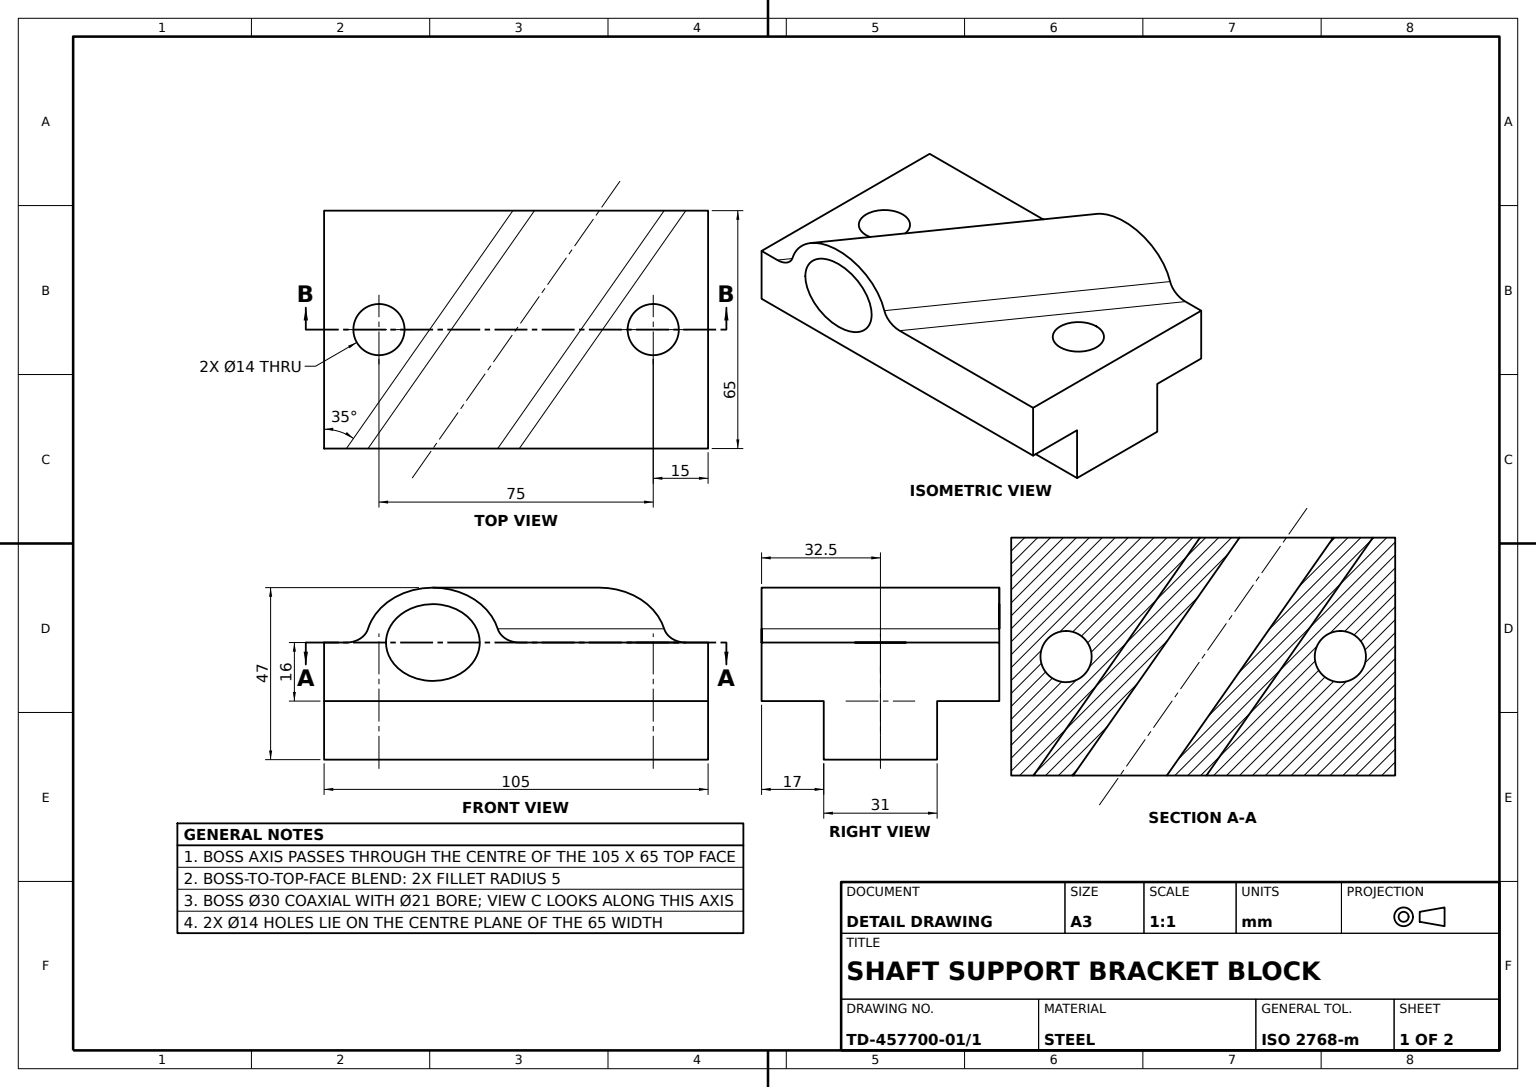
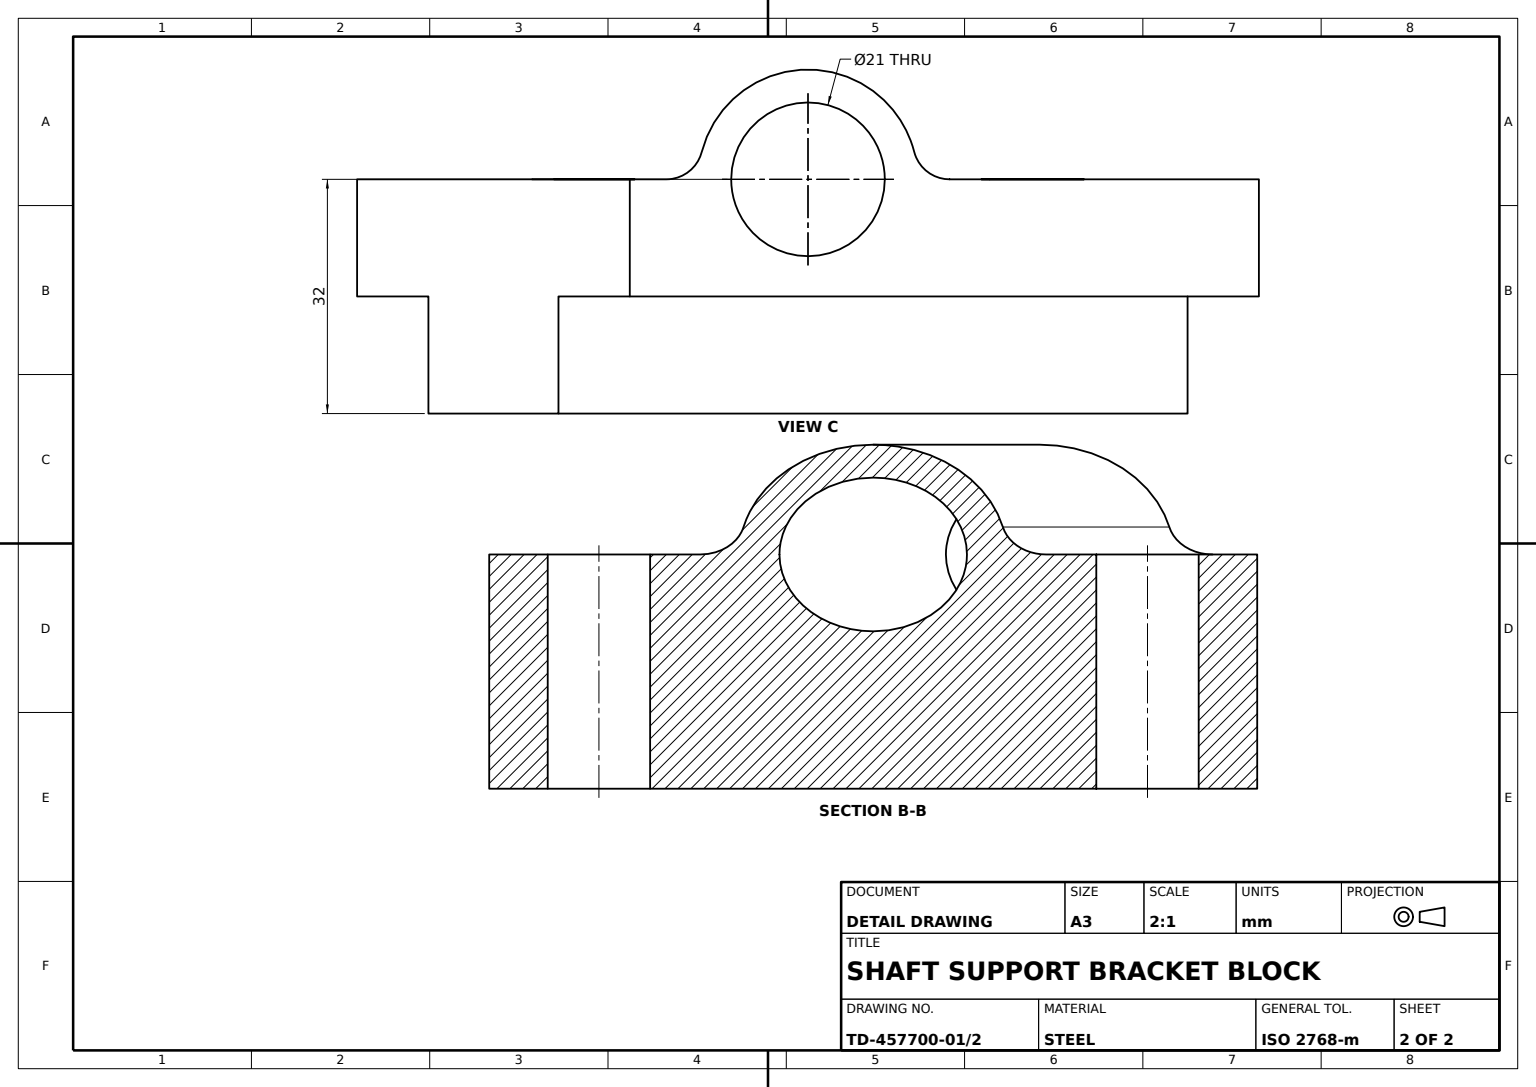
SolidWorks part; units mm, degrees
material "Plain Carbon Steel"
ref_plane "Front Plane" through (0, 0, 0) normal (0, 0, 1) x (1, 0, 0)
ref_plane "Top Plane" through (0, 0, 0) normal (0, 1, 0) x (1, 0, 0)
ref_plane "Right Plane" through (0, 0, 0) normal (1, 0, 0) x (0, 0, -1)
sketch "Base Plate Sketch" plane through (0, 0, 0) normal (0, 1, 0) x (1, 0, 0)
  line L1 (-52.5, -32.5) -> (52.5, -32.5)
  line L2 (-52.5, -32.5) -> (-52.5, 32.5)
  line L3 (-52.5, 32.5) -> (52.5, 32.5)
  line L4 (52.5, -32.5) -> (52.5, 32.5)
  line L5 (-52.5, -32.5) -> (52.5, 32.5) construction
  line L6 (-52.5, 32.5) -> (52.5, -32.5) construction
  point P0 (0, 0)
  dimension "D1" = 105
  dimension "D2" = 65
extrude "Base Plate" add sketch "Base Plate Sketch" against normal blind 16
sketch "Locating Key Sketch" plane through (-52.5, 0, 0) normal (-1, 0, 0) x (0, 0, 1)
  line L0 (-32.5, -16) -> (32.5, -16) construction
  line L1 (-15.5, -16) -> (15.5, -16)
  line L2 (-15.5, -16) -> (-15.5, -32)
  line L3 (-15.5, -32) -> (15.5, -32)
  line L4 (15.5, -16) -> (15.5, -32)
  line L5 (-15.5, -16) -> (15.5, -32) construction
  line L6 (-15.5, -32) -> (15.5, -16) construction
  point P0 (0, -16)
  dimension "D1" = 16
  dimension "D2" = 31
extrude "Locating Key" add sketch "Locating Key Sketch" against normal up to surface (105 mm away) up to face at (52.5, -8, 0)
sketch "Mounting Holes Sketch" plane through (0, 0, 0) normal (0, 1, 0) x (1, 0, 0)
  line L0 (0, 0) -> (0, 20.5485) construction
  circle A0 centre (-37.5, 0) radius 7
  circle A1 centre (37.5, 0) radius 7
  dimension "D1" = 14
  dimension "D2" = 75
extrude "Mounting Holes" cut sketch "Mounting Holes Sketch" against normal through all both and the other way through all
sketch "Boss Angle 35deg Sketch" plane through (0, 0, 0) normal (0, 1, 0) x (1, 0, 0)
  line L0 (0, 0) -> (32.4662, -22.7331) construction
  line L1 (0, 0) -> (38.1074, 0) construction
  dimension "D1" = 35
ref_plane "Plane1" through (0, 0, 0) normal (-0.5736, 0, 0.8192) x (0.8192, 0, 0.5736)
sketch "Boss Profile Sketch" plane through (0, 0, 0) normal (-0.5736, 0, 0.8192) x (0.8192, 0, 0.5736)
  circle A0 centre (0, 0) radius 15
  circle A1 centre (0, 0) radius 10.5
  dimension "D1" = 21
  dimension "D2" = 30
extrude "Inclined Cylinder Boss" add sketch "Boss Profile Sketch" along normal up to surface and the other way up to surface up to face at (0, -8, 32.5) other way up to face at (0, -8, -32.5)
sketch "Boss Bore Sketch" plane through (0, 0, 0) normal (-0.5736, 0, 0.8192) x (0.8192, 0, 0.5736)
  circle A0 centre (0, 0) radius 10.5 construction
  circle A1 centre (0, 0) radius 10.5
extrude "Boss Bore" cut sketch "Boss Bore Sketch" against normal through all both and the other way through all
fillet "Boss Blend Fillet R5" radius 5 2 edges at (-18.3116, 0, 0) (18.3116, 0, 0)
